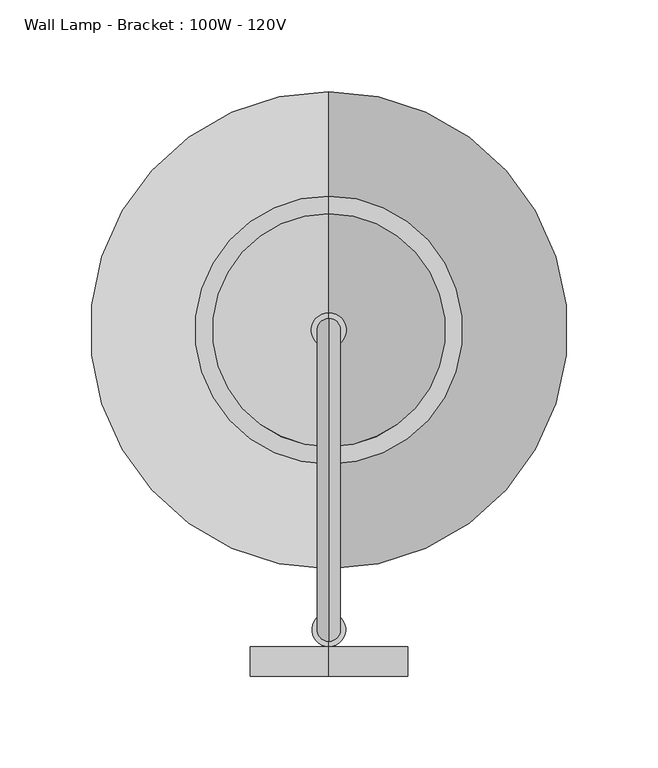
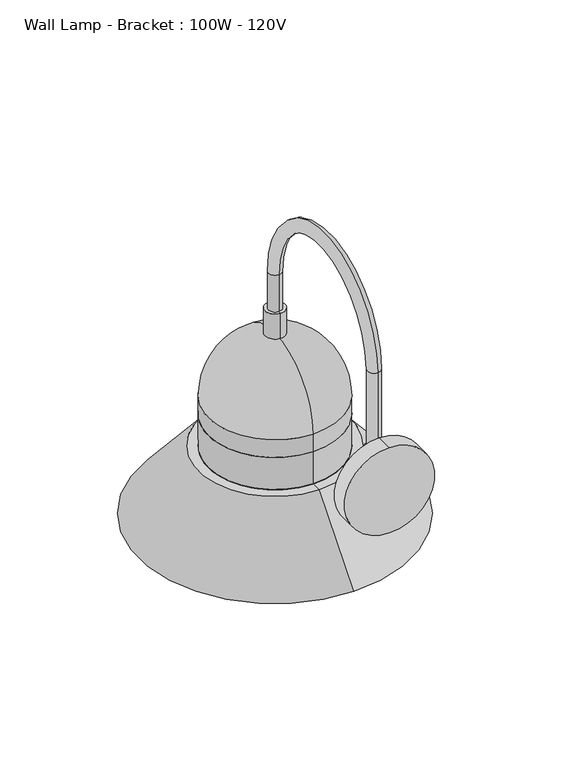
"""IFC4 building model written with IfcOpenShell, lengths in millimetres: light fixture geometry, Wall Lamp - Bracket : 100W - 120V."""

from ifc_helpers import new_model, si_unit, point, frame, frame_2d, origin, place, context, project, spatial, polyline, circle_curve, ellipse_curve, trimmed, segment, composite_curve, outline, extrude, source, transform, mapped, element, save
from ifc_brep_helpers import plane_surface, cylinder_surface, revolved_surface, advanced_brep


def wall_lamp_bracket_100w_120v_38ba4611(model_context):
    return source(origin(), model_context, "Body", "SolidModel", [
        advanced_brep(
        [(-36.3556627, 133.3895413, 2413.7644247), (-36.3556627, 146.0895413, 2413.7644247), (-36.3556627, 146.0895413, 2334.6251468), (-36.3556627, 133.3895413, 2334.6251468), (-36.3556627, 309.5625, 2413.7644247), (-36.3556627, 296.8625, 2413.7644247), (-36.3556627, 309.5625, 2376.6250104), (-36.3556627, 296.8625, 2376.6250104), (-36.3556627, 130.5393793, 2334.6251468), (-36.3556627, 148.9397034, 2334.6251468), (-36.3556627, 148.9397034, 2307.1079598), (-36.3556627, 130.5393793, 2307.1079598), (-36.3556627, 139.7395413, 2297.9077977)],
        [
            (0, 1, circle_curve(frame((-36.3556627, 139.7395413, 2413.7644247), z_axis=(0.0, 0.0, -1.0), x_axis=(0.0, 1.0, 0.0)), 6.35)),
            (1, 2),
            (2, 3, circle_curve(frame((-36.3556627, 139.7395413, 2334.6251468), z_axis=(0.0, 0.0, 1.0), x_axis=(0.0, 1.0, 0.0)), 6.35)),
            (3, 0),
            (1, 0, circle_curve(frame((-36.3556627, 139.7395413, 2413.7644247), z_axis=(0.0, 0.0, -1.0), x_axis=(0.0, 1.0, 0.0)), 6.35)),
            (3, 2, circle_curve(frame((-36.3556627, 139.7395413, 2334.6251468), z_axis=(0.0, 0.0, 1.0), x_axis=(0.0, 1.0, 0.0)), 6.35)),
            (0, 4, circle_curve(frame((-36.3556627, 221.4760207, 2413.7644247), z_axis=(-1.0, 0.0, 0.0), x_axis=(0.0, -1.0, 0.0)), 88.0864793)),
            (4, 5, circle_curve(frame((-36.3556627, 303.2125, 2413.7644247), z_axis=(0.0, 0.0, 1.0), x_axis=(0.0, -1.0, 0.0)), 6.35)),
            (5, 1, circle_curve(frame((-36.3556627, 221.4760207, 2413.7644247), z_axis=(1.0, 0.0, 0.0), x_axis=(0.0, -1.0, 0.0)), 75.3864793)),
            (5, 4, circle_curve(frame((-36.3556627, 303.2125, 2413.7644247), z_axis=(0.0, 0.0, 1.0), x_axis=(0.0, -1.0, 0.0)), 6.35)),
            (6, 7, circle_curve(frame((-36.3556627, 303.2125, 2376.6250104), z_axis=(0.0, 0.0, -1.0), x_axis=(0.0, -1.0, 0.0)), 6.35)),
            (7, 6, circle_curve(frame((-36.3556627, 303.2125, 2376.6250104), z_axis=(0.0, 0.0, -1.0), x_axis=(0.0, -1.0, 0.0)), 6.35)),
            (4, 6),
            (7, 5),
            (8, 9, circle_curve(frame((-36.3556627, 139.7395413, 2334.6251468), z_axis=(0.0, 0.0, 1.0), x_axis=(0.0, -1.0, 0.0)), 9.2001621)),
            (9, 2),
            (3, 8),
            (9, 8, circle_curve(frame((-36.3556627, 139.7395413, 2334.6251468), z_axis=(0.0, 0.0, 1.0), x_axis=(0.0, -1.0, 0.0)), 9.2001621)),
            (10, 11, circle_curve(frame((-36.3556627, 139.7395413, 2307.1079598), z_axis=(0.0, 0.0, -1.0), x_axis=(0.0, -1.0, 0.0)), 9.2001621)),
            (11, 12, circle_curve(frame((-36.3556627, 139.7395413, 2307.1079598), z_axis=(1.0, 0.0, 0.0), x_axis=(0.0, -1.0, 0.0)), 9.2001621)),
            (12, 10, circle_curve(frame((-36.3556627, 139.7395413, 2307.1079598), z_axis=(1.0, 0.0, 0.0), x_axis=(0.0, 1.0, 0.0)), 9.2001621)),
            (11, 10, circle_curve(frame((-36.3556627, 139.7395413, 2307.1079598), z_axis=(0.0, 0.0, -1.0), x_axis=(0.0, -1.0, 0.0)), 9.2001621)),
            (8, 11),
            (10, 9),
        ],
        [
            cylinder_surface(frame((-36.3556627, 139.7395413, 2317.75), z_axis=(0.0, 0.0, -1.0), x_axis=(0.0, 1.0, 0.0)), 6.35),
            revolved_surface(trimmed(ellipse_curve(frame((-36.3556627, 139.7395413, 2413.7644247), z_axis=(0.0, 0.0, -1.0), x_axis=(0.0, 1.0, 0.0)), 6.35, 6.35), [point((-36.3556627, 133.3895413, 2413.7644247))], [point((-36.3556627, 146.0895413, 2413.7644247))], True, "CARTESIAN"), (-36.3556627, 221.4760207, 2413.7644247), (-1.0, 0.0, 0.0)),
            revolved_surface(trimmed(ellipse_curve(frame((-36.3556627, 139.7395413, 2413.7644247), z_axis=(0.0, 0.0, -1.0), x_axis=(0.0, 1.0, 0.0)), 6.35, 6.35), [point((-36.3556627, 146.0895413, 2413.7644247))], [point((-36.3556627, 133.3895413, 2413.7644247))], True, "CARTESIAN"), (-36.3556627, 221.4760207, 2413.7644247), (-1.0, 0.0, 0.0)),
            plane_surface(frame((-36.3556627, 296.8625, 2376.6250104), z_axis=(0.0, 0.0, -1.0), x_axis=(-1.0, 0.0, 0.0))),
            cylinder_surface(frame((-36.3556627, 303.2125, 2413.7644247), z_axis=(0.0, 0.0, 1.0), x_axis=(0.0, -1.0, 0.0)), 6.35),
            plane_surface(frame((-36.3556627, 139.7395413, 2334.6251468), z_axis=(0.0, 0.0, 1.0), x_axis=(0.0, -1.0, 0.0))),
            revolved_surface(trimmed(ellipse_curve(frame((-36.3556627, 139.7395413, 2307.1079598), z_axis=(-1.0, 0.0, 0.0), x_axis=(0.0, -1.0, 0.0)), 9.2001621, 9.2001621), [point((-36.3556627, 139.7395413, 2297.9077977))], [point((-36.3556627, 130.5393793, 2307.1079598))], True, "CARTESIAN"), (-36.3556627, 139.7395413, 2472.7469008), (0.0, 0.0, 1.0)),
            cylinder_surface(frame((-36.3556627, 139.7395413, 2472.7469008), z_axis=(0.0, 0.0, 1.0), x_axis=(0.0, -1.0, 0.0)), 9.2001621),
        ],
        [
            (0, [[1, 2, 3, 4]]),
            (0, [[5, -4, 6, -2]]),
            (1, [[-1, 7, 8, 9]]),
            (2, [[-5, -9, 10, -7]]),
            (3, [[11, 12]]),
            (4, [[-8, 13, -12, 14]]),
            (4, [[-10, -14, -11, -13]]),
            (5, [[15, 16, -6, 17]]),
            (5, [[18, -17, -3, -16]]),
            (6, [[19, 20, 21]]),
            (6, [[-20, 22, -21]]),
            (7, [[-15, 23, -19, 24]]),
            (7, [[-18, -24, -22, -23]]),
        ],
    ),
        extrude(outline(composite_curve([segment(trimmed(circle_curve(frame_2d((2307.1079598, -36.3556627)), 43.0116676), [point((2264.0962922, -36.3556627))], [point((2350.1196273, -36.3556627))], False, "CARTESIAN"), True, "CONTINUOUS"), segment(trimmed(circle_curve(frame_2d((2307.1079598, -36.3556627)), 43.0116676), [point((2350.1196273, -36.3556627))], [point((2264.0962922, -36.3556627))], False, "CARTESIAN"), True, "CONTINUOUS")], self_intersect=False)), frame((0.0, 114.3, 0.0), z_axis=(0.0, 1.0, 0.0), x_axis=(0.0, 0.0, 1.0)), (0.0, 0.0, 1.0), 16.2393793),
        advanced_brep(
        [(-36.3556627, 366.7125, 2237.5701357), (-36.3556627, 239.7125, 2237.5701357), (-36.3556627, 239.7125, 2197.1), (-36.3556627, 366.7125, 2197.1), (-36.3556627, 303.2125, 2237.5701357), (-36.3556627, 303.2125, 2133.6)],
        [
            (0, 1, circle_curve(frame((-36.3556627, 303.2125, 2237.5701357), z_axis=(0.0, 0.0, -1.0), x_axis=(0.0, -1.0, 0.0)), 63.5)),
            (1, 2),
            (2, 3, circle_curve(frame((-36.3556627, 303.2125, 2197.1), z_axis=(0.0, 0.0, 1.0), x_axis=(0.0, -1.0, 0.0)), 63.5)),
            (3, 0),
            (1, 0, circle_curve(frame((-36.3556627, 303.2125, 2237.5701357), z_axis=(0.0, 0.0, -1.0), x_axis=(0.0, -1.0, 0.0)), 63.5)),
            (3, 2, circle_curve(frame((-36.3556627, 303.2125, 2197.1), z_axis=(0.0, 0.0, 1.0), x_axis=(0.0, -1.0, 0.0)), 63.5)),
            (4, 1),
            (0, 4),
            (2, 5, circle_curve(frame((-36.3556627, 303.2125, 2197.1), z_axis=(1.0, 0.0, 0.0), x_axis=(0.0, -1.0, 0.0)), 63.5)),
            (5, 3, circle_curve(frame((-36.3556627, 303.2125, 2197.1), z_axis=(1.0, 0.0, 0.0), x_axis=(0.0, 1.0, 0.0)), 63.5)),
        ],
        [
            cylinder_surface(frame((-36.3556627, 303.2125, -914.4), z_axis=(0.0, 0.0, 1.0), x_axis=(0.0, -1.0, 0.0)), 63.5),
            plane_surface(frame((-36.3556627, 303.2125, 2237.5701357), z_axis=(0.0, 0.0, 1.0), x_axis=(0.0, -1.0, 0.0))),
            revolved_surface(trimmed(ellipse_curve(frame((-36.3556627, 303.2125, 2197.1), z_axis=(-1.0, 0.0, 0.0), x_axis=(0.0, -1.0, 0.0)), 63.5, 63.5), [point((-36.3556627, 303.2125, 2133.6))], [point((-36.3556627, 239.7125, 2197.1))], True, "CARTESIAN"), (-36.3556627, 303.2125, -914.4), (0.0, 0.0, 1.0)),
        ],
        [
            (0, [[1, 2, 3, 4]]),
            (0, [[5, -4, 6, -2]]),
            (1, [[7, -1, 8]]),
            (1, [[-8, -5, -7]]),
            (2, [[-3, 9, 10]]),
            (2, [[-6, -10, -9]]),
        ],
    ),
        advanced_brep(
        [(-36.3556627, 366.7125, 2269.8272766), (-36.3556627, 239.7125, 2269.8272766), (-36.3556627, 239.7125, 2237.5701357), (-36.3556627, 366.7125, 2237.5701357), (-36.3556627, 363.5375, 2269.8272766), (-36.3556627, 242.8875, 2269.8272766), (-36.3556627, 363.5375, 2234.3951357), (-36.3556627, 242.8875, 2234.3951357), (-36.3556627, 374.9669546, 2234.3951357), (-36.3556627, 231.4580454, 2234.3951357), (-36.3556627, 429.247628, 2169.5241129), (-36.3556627, 177.177372, 2169.5241129), (-36.3556627, 433.3875, 2169.5241129), (-36.3556627, 173.0375, 2169.5241129), (-36.3556627, 376.4501529, 2237.5701357), (-36.3556627, 229.9748471, 2237.5701357)],
        [
            (0, 1, circle_curve(frame((-36.3556627, 303.2125, 2269.8272766), z_axis=(0.0, 0.0, -1.0), x_axis=(0.0, -1.0, 0.0)), 63.5)),
            (1, 2),
            (2, 3, circle_curve(frame((-36.3556627, 303.2125, 2237.5701357), z_axis=(0.0, 0.0, 1.0), x_axis=(0.0, -1.0, 0.0)), 63.5)),
            (3, 0),
            (1, 0, circle_curve(frame((-36.3556627, 303.2125, 2269.8272766), z_axis=(0.0, 0.0, -1.0), x_axis=(0.0, -1.0, 0.0)), 63.5)),
            (3, 2, circle_curve(frame((-36.3556627, 303.2125, 2237.5701357), z_axis=(0.0, 0.0, 1.0), x_axis=(0.0, -1.0, 0.0)), 63.5)),
            (4, 5, circle_curve(frame((-36.3556627, 303.2125, 2269.8272766), z_axis=(0.0, 0.0, -1.0), x_axis=(0.0, -1.0, 0.0)), 60.325)),
            (5, 1),
            (0, 4),
            (5, 4, circle_curve(frame((-36.3556627, 303.2125, 2269.8272766), z_axis=(0.0, 0.0, -1.0), x_axis=(0.0, -1.0, 0.0)), 60.325)),
            (6, 7, circle_curve(frame((-36.3556627, 303.2125, 2234.3951357), z_axis=(0.0, 0.0, -1.0), x_axis=(0.0, -1.0, 0.0)), 60.325)),
            (7, 5),
            (4, 6),
            (7, 6, circle_curve(frame((-36.3556627, 303.2125, 2234.3951357), z_axis=(0.0, 0.0, -1.0), x_axis=(0.0, -1.0, 0.0)), 60.325)),
            (8, 9, circle_curve(frame((-36.3556627, 303.2125, 2234.3951357), z_axis=(0.0, 0.0, -1.0), x_axis=(0.0, -1.0, 0.0)), 71.7544546)),
            (9, 7),
            (6, 8),
            (9, 8, circle_curve(frame((-36.3556627, 303.2125, 2234.3951357), z_axis=(0.0, 0.0, -1.0), x_axis=(0.0, -1.0, 0.0)), 71.7544546)),
            (10, 11, circle_curve(frame((-36.3556627, 303.2125, 2169.5241129), z_axis=(0.0, 0.0, -1.0), x_axis=(0.0, -1.0, 0.0)), 126.035128)),
            (11, 9),
            (8, 10),
            (11, 10, circle_curve(frame((-36.3556627, 303.2125, 2169.5241129), z_axis=(0.0, 0.0, -1.0), x_axis=(0.0, -1.0, 0.0)), 126.035128)),
            (12, 13, circle_curve(frame((-36.3556627, 303.2125, 2169.5241129), z_axis=(0.0, 0.0, -1.0), x_axis=(0.0, -1.0, 0.0)), 130.175)),
            (13, 11),
            (10, 12),
            (13, 12, circle_curve(frame((-36.3556627, 303.2125, 2169.5241129), z_axis=(0.0, 0.0, -1.0), x_axis=(0.0, -1.0, 0.0)), 130.175)),
            (14, 15, circle_curve(frame((-36.3556627, 303.2125, 2237.5701357), z_axis=(0.0, 0.0, -1.0), x_axis=(0.0, -1.0, 0.0)), 73.2376529)),
            (15, 13),
            (12, 14),
            (15, 14, circle_curve(frame((-36.3556627, 303.2125, 2237.5701357), z_axis=(0.0, 0.0, -1.0), x_axis=(0.0, -1.0, 0.0)), 73.2376529)),
            (2, 15),
            (14, 3),
        ],
        [
            cylinder_surface(frame((-36.3556627, 303.2125, -914.4), z_axis=(0.0, 0.0, 1.0), x_axis=(0.0, -1.0, 0.0)), 63.5),
            plane_surface(frame((-36.3556627, 303.2125, 2269.8272766), z_axis=(0.0, 0.0, 1.0), x_axis=(0.0, -1.0, 0.0))),
            revolved_surface(polyline([(-36.3556627, 242.8875, 2269.8272766), (-36.3556627, 242.8875, 2234.3951357)]), (-36.3556627, 303.2125, -914.4), (0.0, 0.0, 1.0)),
            plane_surface(frame((-36.3556627, 303.2125, 2234.3951357), z_axis=(0.0, 0.0, -1.0), x_axis=(0.0, -1.0, 0.0))),
            revolved_surface(polyline([(-36.3556627, 231.4580454, 2234.3951357), (-36.3556627, 177.177372, 2169.5241129)]), (-36.3556627, 303.2125, -914.4), (0.0, 0.0, 1.0)),
            plane_surface(frame((-36.3556627, 303.2125, 2169.5241129), z_axis=(0.0, 0.0, -1.0), x_axis=(0.0, -1.0, 0.0))),
            revolved_surface(polyline([(-36.3556627, 173.0375, 2169.5241129), (-36.3556627, 229.9748471, 2237.5701357)]), (-36.3556627, 303.2125, -914.4), (0.0, 0.0, 1.0)),
            plane_surface(frame((-36.3556627, 303.2125, 2237.5701357), z_axis=(0.0, 0.0, 1.0), x_axis=(0.0, -1.0, 0.0))),
        ],
        [
            (0, [[1, 2, 3, 4]]),
            (0, [[5, -4, 6, -2]]),
            (1, [[7, 8, -1, 9]]),
            (1, [[10, -9, -5, -8]]),
            (2, [[11, 12, -7, 13]]),
            (2, [[14, -13, -10, -12]]),
            (3, [[15, 16, -11, 17]]),
            (3, [[18, -17, -14, -16]]),
            (4, [[19, 20, -15, 21]]),
            (4, [[22, -21, -18, -20]]),
            (5, [[23, 24, -19, 25]]),
            (5, [[26, -25, -22, -24]]),
            (6, [[27, 28, -23, 29]]),
            (6, [[30, -29, -26, -28]]),
            (7, [[-3, 31, -27, 32]]),
            (7, [[-6, -32, -30, -31]]),
        ],
    ),
        advanced_brep(
        [(-36.3556627, 366.7125, 2287.7818991), (-36.3556627, 239.7125, 2287.7818991), (-36.3556627, 239.7125, 2269.8272766), (-36.3556627, 366.7125, 2269.8272766), (-36.3556627, 303.2125, 2351.2818991), (-36.3556627, 303.2125, 2269.8272766)],
        [
            (0, 1, circle_curve(frame((-36.3556627, 303.2125, 2287.7818991), z_axis=(0.0, 0.0, -1.0), x_axis=(0.0, -1.0, 0.0)), 63.5)),
            (1, 2),
            (2, 3, circle_curve(frame((-36.3556627, 303.2125, 2269.8272766), z_axis=(0.0, 0.0, 1.0), x_axis=(0.0, -1.0, 0.0)), 63.5)),
            (3, 0),
            (1, 0, circle_curve(frame((-36.3556627, 303.2125, 2287.7818991), z_axis=(0.0, 0.0, -1.0), x_axis=(0.0, -1.0, 0.0)), 63.5)),
            (3, 2, circle_curve(frame((-36.3556627, 303.2125, 2269.8272766), z_axis=(0.0, 0.0, 1.0), x_axis=(0.0, -1.0, 0.0)), 63.5)),
            (4, 1, circle_curve(frame((-36.3556627, 303.2125, 2287.7818991), z_axis=(1.0, 0.0, 0.0), x_axis=(0.0, -1.0, 0.0)), 63.5)),
            (0, 4, circle_curve(frame((-36.3556627, 303.2125, 2287.7818991), z_axis=(1.0, 0.0, 0.0), x_axis=(0.0, 1.0, 0.0)), 63.5)),
            (2, 5),
            (5, 3),
        ],
        [
            cylinder_surface(frame((-36.3556627, 303.2125, -914.4), z_axis=(0.0, 0.0, 1.0), x_axis=(0.0, -1.0, 0.0)), 63.5),
            revolved_surface(trimmed(ellipse_curve(frame((-36.3556627, 303.2125, 2287.7818991), z_axis=(-1.0, 0.0, 0.0), x_axis=(0.0, -1.0, 0.0)), 63.5, 63.5), [point((-36.3556627, 239.7125, 2287.7818991))], [point((-36.3556627, 303.2125, 2351.2818991))], True, "CARTESIAN"), (-36.3556627, 303.2125, -914.4), (0.0, 0.0, 1.0)),
            plane_surface(frame((-36.3556627, 303.2125, 2269.8272766), z_axis=(0.0, 0.0, -1.0), x_axis=(0.0, -1.0, 0.0))),
        ],
        [
            (0, [[1, 2, 3, 4]]),
            (0, [[5, -4, 6, -2]]),
            (1, [[7, -1, 8]]),
            (1, [[-8, -5, -7]]),
            (2, [[-3, 9, 10]]),
            (2, [[-6, -10, -9]]),
        ],
    ),
        advanced_brep(
        [(-36.3556627, 312.7375, 2351.5511541), (-36.3556627, 293.6875, 2351.5511541), (-36.3556627, 303.2125, 2351.5511541), (-36.3556627, 312.7375, 2376.6250104), (-36.3556627, 293.6875, 2376.6250104), (-36.3556627, 303.2125, 2376.6250104)],
        [
            (0, 1, circle_curve(frame((-36.3556627, 303.2125, 2351.5511541), z_axis=(0.0, 0.0, -1.0), x_axis=(0.0, -1.0, 0.0)), 9.525)),
            (1, 2),
            (2, 0),
            (1, 0, circle_curve(frame((-36.3556627, 303.2125, 2351.5511541), z_axis=(0.0, 0.0, -1.0), x_axis=(0.0, -1.0, 0.0)), 9.525)),
            (3, 4, circle_curve(frame((-36.3556627, 303.2125, 2376.6250104), z_axis=(0.0, 0.0, -1.0), x_axis=(0.0, -1.0, 0.0)), 9.525)),
            (4, 1),
            (0, 3),
            (4, 3, circle_curve(frame((-36.3556627, 303.2125, 2376.6250104), z_axis=(0.0, 0.0, -1.0), x_axis=(0.0, -1.0, 0.0)), 9.525)),
            (5, 4),
            (3, 5),
        ],
        [
            plane_surface(frame((-36.3556627, 303.2125, 2351.5511541), z_axis=(0.0, 0.0, -1.0), x_axis=(0.0, -1.0, 0.0))),
            cylinder_surface(frame((-36.3556627, 303.2125, -914.4), z_axis=(0.0, 0.0, 1.0), x_axis=(0.0, -1.0, 0.0)), 9.525),
            plane_surface(frame((-36.3556627, 303.2125, 2376.6250104), z_axis=(0.0, 0.0, 1.0), x_axis=(0.0, -1.0, 0.0))),
        ],
        [
            (0, [[1, 2, 3]]),
            (0, [[4, -3, -2]]),
            (1, [[5, 6, -1, 7]]),
            (1, [[8, -7, -4, -6]]),
            (2, [[9, -5, 10]]),
            (2, [[-10, -8, -9]]),
        ],
    ),
    ])


if __name__ == "__main__":
    model = new_model("IFC4")
    model_context = context("Model", 3, world=origin())
    ifc_project = project(units=[si_unit("LENGTHUNIT", "METRE", prefix="MILLI")], contexts=[model_context])
    site = spatial("IfcSite", under=ifc_project)
    building = spatial("IfcBuilding", under=site)
    placement = place(None, origin())
    wall_lamp_bracket_100w_120v_shape = wall_lamp_bracket_100w_120v_38ba4611(model_context)
    element("IfcLightFixture", 1, ObjectType="Wall Lamp - Bracket : 100W - 120V", at=placement, inside=building, context=model_context, shape_type="MappedRepresentation", body=[
        mapped(wall_lamp_bracket_100w_120v_shape, transform((0.0, 0.0, 0.0), x_axis=(1.0, 0.0, 0.0), y_axis=(0.0, 1.0, 0.0), z_axis=(0.0, 0.0, 1.0))),
    ])
    save(model, "model.ifc")

# Revit data of these elements
# Type "Wall Lamp - Bracket : 100W - 120V"
#   Lamp = "A-19"
#   Assembly Code = "D5020220"
#   Wattage = 100 W
#   built-in parameter 1150110 = 1 (stored number, unit not read)
#   built-in parameter 1114217 = 1 (stored number, unit not read)
#   built-in parameter 1150109 = 1 (stored number, unit not read)
#   built-in parameter 1150113 = 1 (stored number, unit not read)
#   built-in parameter 1150115 = 1 (stored number, unit not read)
#   built-in parameter 1150105 = 134.486 (stored number, unit not read)
#   Light Source Symbol Size = 2' - 0"
#   built-in parameter 1150112 = 1 (stored number, unit not read)
#   built-in parameter 1150114 = 1 (stored number, unit not read)
#   built-in parameter 1150107 = 2800 (stored number, unit not read)
#   built-in parameter 1150106 = 1.34486 (stored number, unit not read)
#   built-in parameter 1150104 = 1.57006 (stored number, unit not read)
#   Ballast Voltage = 120 V
#   built-in parameter 1114218 = 1 (stored number, unit not read)
#   built-in parameter 1150133 = 10 (stored number, unit not read)
#   Lumens = 1690 lm
#   Apparent Load = 100 VA
#   built-in parameter 1150134 = 4
#   built-in parameter 1150137 = 1
#   Color Filter = 16777215
#   built-in parameter 1140040 [instance default] = 1
#   Ballast Number of Poles = 1
#   Bulb Material = Glass, White, High Luminance
#   Shade Material = Glass, Frosted
#   Wall Mount Material = Steel, Chrome Plated
#   Dimming Lamp Color Temperature Shift = (empty or 0)
#   Default Elevation = 0
#   Wattage Comments = ""
# Element 1 (IfcLightFixture, "Wall Lamp - Bracket : 100W - 120V")
#   Materials on its faces: "Steel, Chrome Plated", "Glass, Frosted", "Glass, White, High Luminance"
# Materials
#   "Glass, White, High Luminance": class "Glass", colour RGB 249 250 249, transparency 0.8, Description = "physical material", Cost = 0
#   "Glass, Frosted": class "Glass", colour RGB 250 244 225, transparency 0.55, Description = "physical material", Cost = 0
#   "Steel, Chrome Plated": class "Metal", colour RGB 17 17 17, transparency 0, Description = "Chromiuim plated steel", Cost = 0
